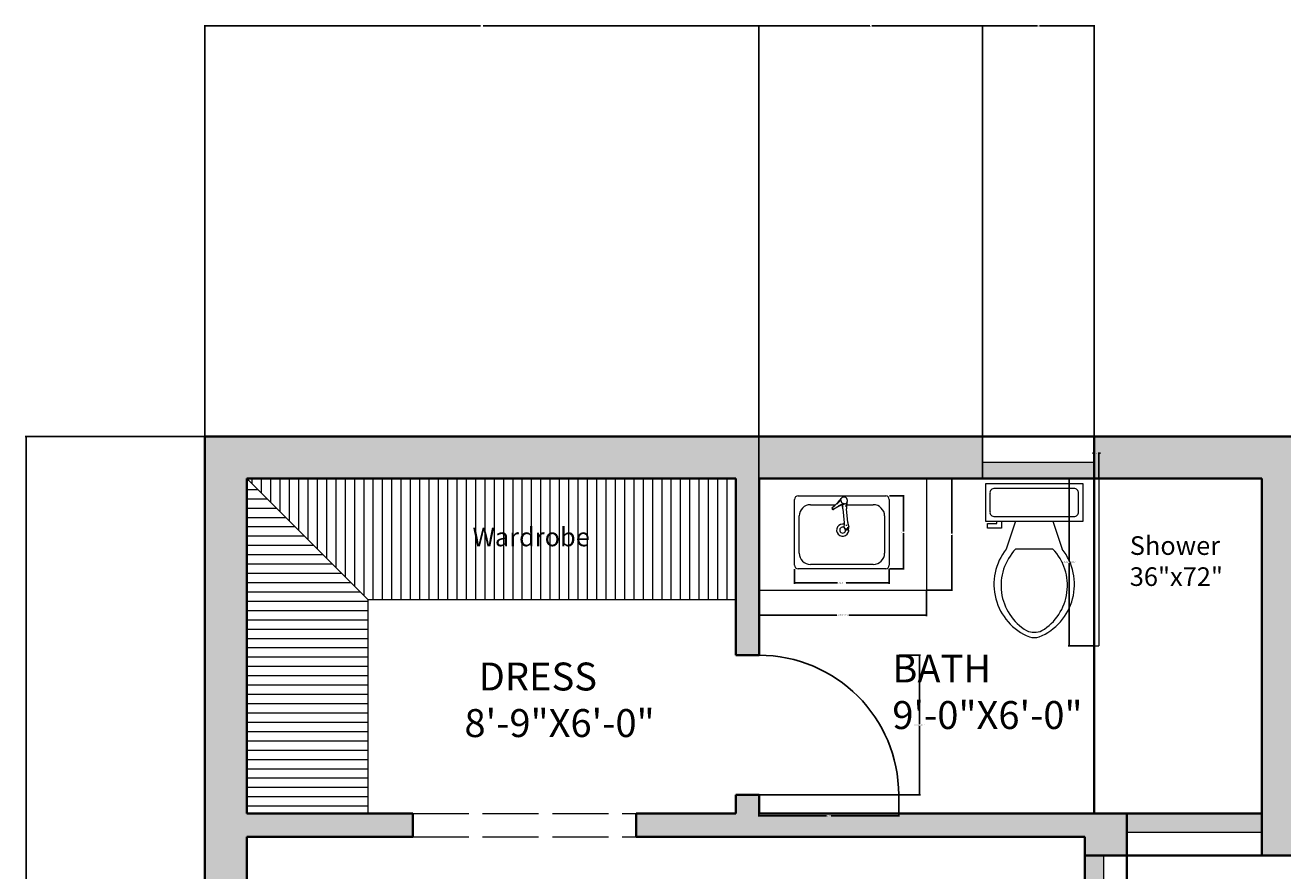
# Model space of a CAD drawing. Units: inches. Extents: x 2985 to 3527, y 3685 to 4528.
# Tile 4 of 5: x 2985 to 3255, y 4346 to 4528. Entities that reach past the tile are written whole.
import ezdxf

# ---------------------------------------------------------------- set-up
doc = ezdxf.new("R2010")
doc.units = ezdxf.units.IN
doc.linetypes.add('ACAD_ISO02W100', pattern=[15, 12, -3])
for name, color, linetype, lineweight in [('A-ANNO-DIMS', 2, 'Continuous', 18), ('A-ANNO-TEXT', 7, 'Continuous', 18), ('A-AREA-IDEN', 7, 'Continuous', 25), ('A-FLOR-CASE', 9, 'Continuous', 20), ('A-FLOR-CASE-PATT', 9, 'Continuous', 13), ('A-FLOR-FIXT', 9, 'Continuous', 18), ('A-GLAZ', 4, 'Continuous', 18), ('A-WALL', 7, 'Continuous', 40), ('A-WALL-OVHD', 7, 'ACAD_ISO02W100', 18), ('A-WALL-PATT', 8, 'Continuous', 13), ('door', 4, 'Continuous', 25)]:
    doc.layers.add(name, color=color, linetype=linetype, lineweight=lineweight)
doc.layers.add('A-GLAZ-PATT', color=241, linetype='Continuous', lineweight=13, true_color=0xf7abae)
doc.styles.get("Standard").update_dxf_attribs({"font": 'arial.ttf'})
doc.dimstyles.get("Standard").update_dxf_attribs({"dimtxt": 0.18, "dimasz": 0.18, "dimexe": 0.18, "dimexo": 0.0625, "dimgap": 0.09, "dimtad": 0, "dimtih": 1, "dimtoh": 1, "dimdec": 4, "dimzin": 0, "dimdsep": 46, "dimtxsty": 'Standard', "dimcen": 0.09, "dimadec": 0, "dimazin": 0, "dimtfac": 1, "dimtdec": 4, "dimtofl": 0, "dimtmove": 0, "dimatfit": 3, "dimfxl": 1, "dimtolj": 1, "dimtzin": 0, "dimarcsym": 0})

# ---------------------------------------------------------------- blocks, each defined once
blk = doc.blocks.new('*U2')
for p, q in [((9.5, -6), (9.5, -2)), ((-8, -8.5), (-8, -8)), ((-7, -8), (-7, -9.5)), ((-4, -8), (-6, -14)), ((4, -8), (6, -14)), ((-10, -8.5), (-8, -8.5)), ((-10, -9.5), (-10, -8.5)), ((-7, -9.5), (-10, -9.5)), ((4, -14), (-4, -14))]:
    blk.add_line(p, q)
blk.add_lwpolyline([(10.5, -8), (10.5, 0), (-10.5, 0), (-10.5, -8)], close=True)
for points in [[(-9.5, -2), (-9.5, -6)], [(8.5, -1), (-8.5, -1)], [(-8.5, -7), (8.5, -7)]]:
    blk.add_lwpolyline(points)
for centre, radius, start, end in [((-8.62, -1.88), 0.884, 81.8699, 188.1301), ((8.62, -1.88), 0.884, 351.8699, 98.1301), ((-8.62, -6.12), 0.884, 171.8699, 278.1301), ((8.62, -6.12), 0.884, 261.8699, 8.1301), ((3.52, -21.58), 12.17, 141.4691, 247.9714), ((4.2, -21.82), 11.33, 136.3677, 238.9468), ((-3.52, -21.58), 12.17, 292.0284, 38.5307), ((-4.2, -21.82), 11.33, 301.053, 43.6321), ((0, -27.88), 4, 245.7318, 294.2682), ((0, -29), 4, 254.8605, 285.1395)]:
    blk.add_arc(centre, radius, start, end)
blk = doc.blocks.new('A$C1B254B08')
for p, q in [((0, 20), (0, 394.5)), ((20, 414.5), (278.5, 414.5)), ((90.2, 364.5), (232.9, 364.5)), ((278.5, 414.5), (518, 414.5)), ((296.4, 364.5), (447.8, 364.5)), ((538, 394.5), (538, 20)), ((26.2, 88.5), (26.2, 300.5)), ((275, 340.3), (282.6, 261.9)), ((303, 263.9), (295.5, 341.4)), ((511.8, 300.5), (511.8, 88.5)), ((447.8, 24.5), (90.2, 24.5)), ((518, 0), (20, 0))]:
    blk.add_line(p, q)
for centre, radius, start, end in [((20, 394.5), 20, 90, 180), ((90.2, 300.5), 64, 90, 180), ((59.9, 551.8), 255, 307.29995, 323.44123), ((362.9, 125.6), 255, 107.37848, 123.51976), ((189.9, 438.1), 86.6, 305.66886, 327.17012), ((298.2, 285.8), 86.6, 103.6496, 125.15085), ((280, 388.4), 16.2, 164.00843, 277.23501), ((280.7, 388), 20, 287.37848, 143.44123), ((175.5, 330.4), 100, 5.6774, 19.04527), ((246.9, 349.5), 29.3, 4.17107, 27.91331), ((320.7, 356.3), 29.3, 157.81042, 186.31744), ((395, 351.3), 100, 162.19035, 185.67746), ((447.8, 300.5), 64, 0, 90), ((518, 394.5), 20, 0, 90), ((218.4, 343.7), 6.64, 127.29995, 303.51976), ((220.3, 343.9), 4.91, 158.92924, 241.9125), ((273.7, 220.2), 34.6, 74.3543, 12.13808), ((273.7, 220.2), 16.8, 61.4601, 4.85789), ((295.6, 234.6), 13.9, 171.17496, 20.1799), ((183.1, 252), 100, 351.17496, 5.6774), ((295.7, 235), 8.12, 213.71984, 15.80061), ((295.2, 239.5), 7.59, 64.48838, 123.74119), ((402.5, 273.8), 100, 185.67746, 200.1799), ((90.2, 88.5), 64, 180, 270), ((447.8, 88.5), 64, 270, 0), ((20, 20), 20, 180, 270), ((518, 20), 20, 270, 0)]:
    blk.add_arc(centre, radius, start, end)
blk = doc.blocks.new('DOOR-SWING-30IN')
blk.add_line((0, 0), (30, 0))
blk.add_arc((0, 0), 30, 0, 90)
blk = doc.blocks.new('SHOWER-SCREEN-36IN')
for p in [(1, 36), (0, 0)]:
    blk.add_line(p, (1, 0))
blk = doc.blocks.new('VANITY-TOP-36X24IN')
for p in [(36, 24), (0, 0)]:
    blk.add_line(p, (36, 0))
blk = doc.blocks.new('*D20')
at = {"layer": 'A-ANNO-DIMS', "color": 0, "lineweight": -2, "transparency": 16777216}
for p, q in [((3172.9, 4392.37), (3177.51, 4392.37)), ((3177.33, 4392.19), (3177.33, 4377.56)), ((3177.33, 4362.55), (3177.33, 4377.19)), ((3172.9, 4362.37), (3177.51, 4362.37))]:
    blk.add_line(p, q, dxfattribs=at)
at = {"layer": 'A-ANNO-DIMS', "color": 0, "transparency": 16777216}
for points in [[(3177.3, 4392.19), (3177.36, 4392.19), (3177.33, 4392.37)], [(3177.3, 4362.55), (3177.36, 4362.55), (3177.33, 4362.37)]]:
    blk.add_solid(points, dxfattribs=at)
at = {"layer": 'Defpoints', "color": 0, "transparency": 16777216}
for p in [(3172.83, 4392.37), (3177.33, 4392.37), (3172.83, 4362.37)]:
    blk.add_point(p, dxfattribs=at)
at = {"layer": 'A-ANNO-DIMS', "color": 0, "transparency": 16777216, "insert": (3177.33, 4377.37), "char_height": 0.18, "attachment_point": 5}
blk.add_mtext('\\A1;BATH DOOR 30 TYP.', dxfattribs=at)
blk = doc.blocks.new('*D21')
at = {"layer": 'A-ANNO-DIMS', "color": 0, "lineweight": -2, "transparency": 16777216}
for p, q in [((3142.83, 4362.31), (3142.83, 4357.69)), ((3172.83, 4362.31), (3172.83, 4357.69)), ((3143.01, 4357.87), (3157.31, 4357.87)), ((3172.65, 4357.87), (3158.36, 4357.87))]:
    blk.add_line(p, q, dxfattribs=at)
at = {"layer": 'A-ANNO-DIMS', "color": 0, "transparency": 16777216}
for points in [[(3143.01, 4357.9), (3143.01, 4357.84), (3142.83, 4357.87)], [(3172.65, 4357.9), (3172.65, 4357.84), (3172.83, 4357.87)]]:
    blk.add_solid(points, dxfattribs=at)
at = {"layer": 'Defpoints', "color": 0, "transparency": 16777216}
for p in [(3142.83, 4362.37), (3172.83, 4362.37), (3172.83, 4357.87)]:
    blk.add_point(p, dxfattribs=at)
at = {"layer": 'A-ANNO-DIMS', "color": 0, "transparency": 16777216, "insert": (3157.83, 4357.87), "char_height": 0.18, "attachment_point": 5}
blk.add_mtext('\\A1;30 TYP.', dxfattribs=at)
blk = doc.blocks.new('*D22')
at = {"layer": 'A-ANNO-DIMS', "color": 0, "lineweight": -2, "transparency": 16777216}
for p, q in [((3150.47, 4410.88), (3150.47, 4407.72)), ((3170.79, 4410.88), (3170.79, 4407.72)), ((3150.65, 4407.9), (3159.69, 4407.9)), ((3170.61, 4407.9), (3161.56, 4407.9))]:
    blk.add_line(p, q, dxfattribs=at)
at = {"layer": 'A-ANNO-DIMS', "color": 0, "transparency": 16777216}
for points in [[(3150.65, 4407.93), (3150.65, 4407.87), (3150.47, 4407.9)], [(3170.61, 4407.93), (3170.61, 4407.87), (3170.79, 4407.9)]]:
    blk.add_solid(points, dxfattribs=at)
at = {"layer": 'Defpoints', "color": 0, "transparency": 16777216}
for p in [(3150.47, 4410.95), (3170.79, 4410.95), (3170.79, 4407.9)]:
    blk.add_point(p, dxfattribs=at)
at = {"layer": 'A-ANNO-DIMS', "color": 0, "transparency": 16777216, "insert": (3160.63, 4407.9), "char_height": 0.18, "attachment_point": 5}
blk.add_mtext('\\A1;BASIN 20 TYP.', dxfattribs=at)
blk = doc.blocks.new('*D23')
at = {"layer": 'A-ANNO-DIMS', "color": 0, "lineweight": -2, "transparency": 16777216}
for p, q in [((3170.85, 4426.61), (3174.02, 4426.61)), ((3173.84, 4426.43), (3173.84, 4418.96)), ((3173.84, 4411.13), (3173.84, 4418.59)), ((3170.85, 4410.95), (3174.02, 4410.95))]:
    blk.add_line(p, q, dxfattribs=at)
at = {"layer": 'A-ANNO-DIMS', "color": 0, "transparency": 16777216}
for points in [[(3173.81, 4426.43), (3173.87, 4426.43), (3173.84, 4426.61)], [(3173.81, 4411.13), (3173.87, 4411.13), (3173.84, 4410.95)]]:
    blk.add_solid(points, dxfattribs=at)
at = {"layer": 'Defpoints', "color": 0, "transparency": 16777216}
for p in [(3170.79, 4426.61), (3173.84, 4426.61), (3170.79, 4410.95)]:
    blk.add_point(p, dxfattribs=at)
at = {"layer": 'A-ANNO-DIMS', "color": 0, "transparency": 16777216, "insert": (3173.84, 4418.78), "char_height": 0.18, "attachment_point": 5}
blk.add_mtext('\\A1;16 TYP.', dxfattribs=at)
blk = doc.blocks.new('*D26')
at = {"layer": 'A-ANNO-DIMS', "color": 0, "lineweight": -2, "transparency": 16777216}
for p, q in [((3214.77, 4430.37), (3209.25, 4430.37)), ((3209.43, 4430.19), (3209.43, 4412.56)), ((3209.43, 4394.55), (3209.43, 4412.19)), ((3214.77, 4394.37), (3209.25, 4394.37))]:
    blk.add_line(p, q, dxfattribs=at)
at = {"layer": 'A-ANNO-DIMS', "color": 0, "transparency": 16777216}
for points in [[(3209.4, 4430.19), (3209.46, 4430.19), (3209.43, 4430.37)], [(3209.4, 4394.55), (3209.46, 4394.55), (3209.43, 4394.37)]]:
    blk.add_solid(points, dxfattribs=at)
at = {"layer": 'Defpoints', "color": 0, "transparency": 16777216}
for p in [(3209.43, 4430.37), (3214.83, 4430.37), (3214.83, 4394.37)]:
    blk.add_point(p, dxfattribs=at)
at = {"layer": 'A-ANNO-DIMS', "color": 0, "transparency": 16777216, "insert": (3209.43, 4412.37), "char_height": 0.18, "attachment_point": 5}
blk.add_mtext('\\A1;SHOWER SCREEN 36 TYP.', dxfattribs=at)
blk = doc.blocks.new('*D27')
at = {"layer": 'A-ANNO-DIMS', "color": 0, "lineweight": -2, "transparency": 16777216}
for p, q in [((3214.65, 4435.77), (3214.47, 4435.77)), ((3214.83, 4430.43), (3214.83, 4435.95)), ((3215.83, 4430.43), (3215.83, 4435.95)), ((3216.01, 4435.77), (3216.19, 4435.77))]:
    blk.add_line(p, q, dxfattribs=at)
at = {"layer": 'A-ANNO-DIMS', "color": 0, "transparency": 16777216}
for points in [[(3214.65, 4435.8), (3214.65, 4435.74), (3214.83, 4435.77)], [(3216.01, 4435.8), (3216.01, 4435.74), (3215.83, 4435.77)]]:
    blk.add_solid(points, dxfattribs=at)
at = {"layer": 'Defpoints', "color": 0, "transparency": 16777216}
for p in [(3215.83, 4435.77), (3214.83, 4430.37), (3215.83, 4430.37)]:
    blk.add_point(p, dxfattribs=at)
at = {"layer": 'A-ANNO-DIMS', "color": 0, "transparency": 16777216, "insert": (3215.33, 4435.77), "char_height": 0.18, "attachment_point": 5}
blk.add_mtext('\\A1;1 TYP.', dxfattribs=at)
blk = doc.blocks.new('*D28')
at = {"layer": 'A-ANNO-DIMS', "color": 0, "lineweight": -2, "transparency": 16777216}
for p, q in [((3142.83, 4406.31), (3142.83, 4400.79)), ((3178.83, 4406.31), (3178.83, 4400.79)), ((3143.01, 4400.97), (3159.52, 4400.97)), ((3178.65, 4400.97), (3162.15, 4400.97))]:
    blk.add_line(p, q, dxfattribs=at)
at = {"layer": 'A-ANNO-DIMS', "color": 0, "transparency": 16777216}
for points in [[(3143.01, 4401), (3143.01, 4400.94), (3142.83, 4400.97)], [(3178.65, 4401), (3178.65, 4400.94), (3178.83, 4400.97)]]:
    blk.add_solid(points, dxfattribs=at)
at = {"layer": 'Defpoints', "color": 0, "transparency": 16777216}
for p in [(3142.83, 4406.37), (3178.83, 4406.37), (3178.83, 4400.97)]:
    blk.add_point(p, dxfattribs=at)
at = {"layer": 'A-ANNO-DIMS', "color": 0, "transparency": 16777216, "insert": (3160.83, 4400.97), "char_height": 0.18, "attachment_point": 5}
blk.add_mtext('\\A1;VANITY TOP 36 TYP.', dxfattribs=at)
blk = doc.blocks.new('*D29')
at = {"layer": 'A-ANNO-DIMS', "color": 0, "lineweight": -2, "transparency": 16777216}
for p, q in [((3178.9, 4430.37), (3184.41, 4430.37)), ((3184.23, 4430.19), (3184.23, 4418.55)), ((3184.23, 4406.55), (3184.23, 4418.19)), ((3178.9, 4406.37), (3184.41, 4406.37))]:
    blk.add_line(p, q, dxfattribs=at)
at = {"layer": 'A-ANNO-DIMS', "color": 0, "transparency": 16777216}
for points in [[(3184.2, 4430.19), (3184.26, 4430.19), (3184.23, 4430.37)], [(3184.2, 4406.55), (3184.26, 4406.55), (3184.23, 4406.37)]]:
    blk.add_solid(points, dxfattribs=at)
at = {"layer": 'Defpoints', "color": 0, "transparency": 16777216}
for p in [(3178.83, 4430.37), (3184.23, 4430.37), (3178.83, 4406.37)]:
    blk.add_point(p, dxfattribs=at)
at = {"layer": 'A-ANNO-DIMS', "color": 0, "transparency": 16777216, "insert": (3184.23, 4418.37), "char_height": 0.18, "attachment_point": 5}
blk.add_mtext('\\A1;24 TYP.', dxfattribs=at)
blk = doc.blocks.new('*D41')
at = {"layer": 'A-ANNO-DIMS', "color": 0, "lineweight": -2, "transparency": 16777216}
for p, q in [((3023.77, 4439.37), (2985.25, 4439.37)), ((2985.43, 4439.19), (2985.43, 4081.55)), ((2985.43, 3723.55), (2985.43, 4081.19)), ((3023.77, 3723.37), (2985.25, 3723.37))]:
    blk.add_line(p, q, dxfattribs=at)
at = {"layer": 'A-ANNO-DIMS', "color": 0, "transparency": 16777216}
for points in [[(2985.4, 4439.19), (2985.46, 4439.19), (2985.43, 4439.37)], [(2985.4, 3723.55), (2985.46, 3723.55), (2985.43, 3723.37)]]:
    blk.add_solid(points, dxfattribs=at)
at = {"layer": 'Defpoints', "color": 0, "transparency": 16777216}
for p in [(2985.43, 4439.37), (3023.83, 4439.37), (3023.83, 3723.37)]:
    blk.add_point(p, dxfattribs=at)
at = {"layer": 'A-ANNO-DIMS', "color": 0, "transparency": 16777216, "insert": (2985.43, 4081.37), "char_height": 0.18, "attachment_point": 5}
blk.add_mtext('\\A1;716', dxfattribs=at)
blk = doc.blocks.new('*D46')
at = {"layer": 'A-ANNO-DIMS', "color": 0, "lineweight": -2, "transparency": 16777216}
for p, q in [((3023.83, 4439.43), (3023.83, 4527.76)), ((3024.01, 4527.58), (3083.05, 4527.58)), ((3142.65, 4527.58), (3083.61, 4527.58)), ((3142.83, 4430.43), (3142.83, 4527.76))]:
    blk.add_line(p, q, dxfattribs=at)
at = {"layer": 'A-ANNO-DIMS', "color": 0, "transparency": 16777216}
for points in [[(3024.01, 4527.61), (3024.01, 4527.55), (3023.83, 4527.58)], [(3142.65, 4527.61), (3142.65, 4527.55), (3142.83, 4527.58)]]:
    blk.add_solid(points, dxfattribs=at)
at = {"layer": 'Defpoints', "color": 0, "transparency": 16777216}
for p in [(3142.83, 4527.58), (3023.83, 4439.37), (3142.83, 4430.37)]:
    blk.add_point(p, dxfattribs=at)
at = {"layer": 'A-ANNO-DIMS', "color": 0, "transparency": 16777216, "insert": (3083.33, 4527.58), "char_height": 0.18, "attachment_point": 5}
blk.add_mtext('\\A1;119', dxfattribs=at)
blk = doc.blocks.new('*D47')
at = {"layer": 'A-ANNO-DIMS', "color": 0, "lineweight": -2, "transparency": 16777216}
for p, q in [((3190.83, 4439.43), (3190.83, 4527.76)), ((3191.01, 4527.58), (3202.61, 4527.58)), ((3214.65, 4527.58), (3203.05, 4527.58)), ((3214.83, 4439.43), (3214.83, 4527.76))]:
    blk.add_line(p, q, dxfattribs=at)
at = {"layer": 'A-ANNO-DIMS', "color": 0, "transparency": 16777216}
for points in [[(3191.01, 4527.61), (3191.01, 4527.55), (3190.83, 4527.58)], [(3214.65, 4527.61), (3214.65, 4527.55), (3214.83, 4527.58)]]:
    blk.add_solid(points, dxfattribs=at)
at = {"layer": 'Defpoints', "color": 0, "transparency": 16777216}
for p in [(3214.83, 4527.58), (3190.83, 4439.37), (3214.83, 4439.37)]:
    blk.add_point(p, dxfattribs=at)
at = {"layer": 'A-ANNO-DIMS', "color": 0, "transparency": 16777216, "insert": (3202.83, 4527.58), "char_height": 0.18, "attachment_point": 5}
blk.add_mtext('\\A1;24', dxfattribs=at)
blk = doc.blocks.new('*D50')
at = {"layer": 'A-ANNO-DIMS', "color": 0, "lineweight": -2, "transparency": 16777216}
for p, q in [((3142.83, 4430.43), (3142.83, 4527.76)), ((3143.01, 4527.58), (3166.61, 4527.58)), ((3190.65, 4527.58), (3167.06, 4527.58)), ((3190.83, 4430.43), (3190.83, 4527.76))]:
    blk.add_line(p, q, dxfattribs=at)
at = {"layer": 'A-ANNO-DIMS', "color": 0, "transparency": 16777216}
for points in [[(3143.01, 4527.61), (3143.01, 4527.55), (3142.83, 4527.58)], [(3190.65, 4527.61), (3190.65, 4527.55), (3190.83, 4527.58)]]:
    blk.add_solid(points, dxfattribs=at)
at = {"layer": 'Defpoints', "color": 0, "transparency": 16777216}
for p in [(3190.83, 4527.58), (3142.83, 4430.37), (3190.83, 4430.37)]:
    blk.add_point(p, dxfattribs=at)
at = {"layer": 'A-ANNO-DIMS', "color": 0, "transparency": 16777216, "insert": (3166.83, 4527.58), "char_height": 0.18, "attachment_point": 5}
blk.add_mtext('\\A1;48', dxfattribs=at)

msp = doc.modelspace()

# ---------------------------------------------------------------- hatches: boundary and pattern name
at = {"layer": 'A-FLOR-CASE-PATT'}
h = msp.add_hatch(dxfattribs=at)
h.set_pattern_fill('ANSI31', color=256, scale=0.6299213, angle=-45, style=0)
h.paths.add_polyline_path([(3032.833, 4358.372), (3058.833, 4358.372), (3058.833, 4404.372), (3032.833, 4430.372)])
h = msp.add_hatch(dxfattribs=at)
h.set_pattern_fill('ANSI31', color=256, scale=0.6299213, angle=45, style=0)
h.paths.add_polyline_path([(3032.833, 4430.372), (3058.833, 4404.372), (3137.833, 4404.372), (3137.833, 4430.372)])
at = {"layer": 'A-GLAZ-PATT'}
h = msp.add_hatch(color=256, dxfattribs=at)
h.dxf.hatch_style = 1
h.paths.add_polyline_path([(3214.833, 4433.872), (3190.833, 4433.872), (3190.833, 4430.372), (3214.833, 4430.372)])
h = msp.add_hatch(color=256, dxfattribs=at)
h.dxf.hatch_style = 1
h.paths.add_polyline_path([(3216.833, 4349.372), (3212.833, 4349.372), (3212.833, 4271.372), (3216.833, 4271.372)])
h.paths.add_polyline_path([(3250.833, 4358.372), (3221.833, 4358.372), (3221.833, 4354.372), (3250.833, 4354.372)])
h.paths.add_polyline_path([(3290.333, 4358.372), (3259.833, 4358.372), (3259.833, 4354.372), (3290.333, 4354.372)])
h.paths.add_polyline_path([(3299.333, 4349.372), (3295.333, 4349.372), (3295.333, 4271.372), (3299.333, 4271.372)])
h.paths.add_polyline_path([(3290.333, 4265.372), (3221.833, 4265.372), (3221.833, 4260.372), (3290.333, 4260.372)])
at = {"layer": 'A-WALL-PATT'}
h = msp.add_hatch(color=256, dxfattribs=at)
h.dxf.hatch_style = 1
h.paths.add_polyline_path([(3023.833, 4065.372), (3023.833, 3771.372), (3111.083, 3771.372), (3111.083, 3780.372), (3032.833, 3780.372), (3032.833, 3936.372), (3221.333, 3936.372), (3221.333, 3945.372), (3215.333, 3945.372), (3215.333, 3981.372), (3206.333, 3981.372), (3206.333, 3945.372), (3032.833, 3945.372), (3032.833, 4065.372), (3079.333, 4065.372), (3079.333, 4074.372), (3032.833, 4074.372), (3032.833, 4188.372), (3119.333, 4188.372), (3119.333, 4107.372), (3215.333, 4107.372), (3215.333, 4148.372), (3206.333, 4148.372), (3206.333, 4116.372), (3124.333, 4116.372), (3124.333, 4188.372), (3206.333, 4188.372), (3206.333, 4184.372), (3215.333, 4184.372), (3215.333, 4188.372), (3221.833, 4188.372), (3221.833, 4201.372), (3212.833, 4201.372), (3212.833, 4197.372), (3032.833, 4197.372), (3032.833, 4353.372), (3068.479, 4353.372), (3068.479, 4358.372), (3032.833, 4358.372), (3032.833, 4430.372), (3137.833, 4430.372), (3137.833, 4404.372), (3137.833, 4392.372), (3142.833, 4392.372), (3142.833, 4430.372), (3190.833, 4430.372), (3190.833, 4439.372), (3023.833, 4439.372)])
h = msp.add_hatch(color=256, dxfattribs=at)
h.dxf.hatch_style = 1
h.paths.add_polyline_path([(3259.833, 4430.372), (3295.833, 4430.372), (3295.833, 4439.372), (3214.833, 4439.372), (3214.833, 4430.372), (3250.833, 4430.372), (3250.833, 4349.372), (3259.833, 4349.372)])
h = msp.add_hatch(color=256, dxfattribs=at)
h.dxf.hatch_style = 1
h.paths.add_polyline_path([(3221.833, 4358.372), (3142.833, 4358.372), (3142.833, 4362.372), (3137.833, 4362.372), (3137.833, 4358.372), (3116.479, 4358.372), (3116.479, 4353.372), (3212.833, 4353.372), (3212.833, 4349.372), (3221.833, 4349.372)])

# ---------------------------------------------------------------- linework, layer by layer
at = {"layer": 'A-FLOR-CASE'}
for q in [(3032.833, 4430.372), (3137.833, 4404.372), (3058.833, 4358.372)]:
    msp.add_line((3058.833, 4404.372), q, dxfattribs=at)
at = {"layer": 'A-GLAZ'}
for p, q in [((3190.833, 4439.372), (3190.833, 4430.372)), ((3190.833, 4433.872), (3214.833, 4433.872)), ((3221.833, 4354.372), (3250.833, 4354.372)), ((3216.833, 4349.372), (3216.833, 4271.372))]:
    msp.add_line(p, q, dxfattribs=at)
at = {"layer": 'A-WALL'}
for p, q in [((3023.833, 4439.372), (3023.833, 4065.372)), ((3023.833, 4439.372), (3488.333, 4439.372)), ((3214.833, 4439.372), (3214.833, 4358.372)), ((3032.833, 4430.372), (3032.833, 4358.372)), ((3032.833, 4430.372), (3137.833, 4430.372)), ((3137.833, 4430.372), (3137.833, 4404.372)), ((3142.833, 4430.372), (3142.833, 4392.372)), ((3142.833, 4430.372), (3250.833, 4430.372)), ((3250.833, 4430.372), (3250.833, 4349.372)), ((3137.833, 4404.372), (3137.833, 4392.372)), ((3142.833, 4392.372), (3137.833, 4392.372)), ((3142.833, 4362.372), (3137.833, 4362.372)), ((3137.833, 4362.372), (3137.833, 4358.372)), ((3142.833, 4362.372), (3142.833, 4358.372)), ((3032.833, 4358.372), (3068.479, 4358.372)), ((3068.479, 4358.372), (3068.479, 4353.372)), ((3116.479, 4358.372), (3116.479, 4353.372)), ((3116.479, 4358.372), (3137.833, 4358.372)), ((3142.833, 4358.372), (3250.833, 4358.372)), ((3221.833, 4358.372), (3221.833, 4237.372)), ((3032.833, 4353.372), (3068.479, 4353.372)), ((3032.833, 4353.372), (3032.833, 4197.372)), ((3116.479, 4353.372), (3212.833, 4353.372)), ((3212.833, 4353.372), (3212.833, 4237.372)), ((3212.833, 4349.372), (3299.333, 4349.372))]:
    msp.add_line(p, q, dxfattribs=at)
at = {"layer": 'A-WALL-OVHD'}
for p, q in [((3068.479, 4358.372), (3116.479, 4358.372)), ((3068.479, 4353.372), (3116.479, 4353.372))]:
    msp.add_line(p, q, dxfattribs=at)

# ---------------------------------------------------------------- block references
at = {"layer": 'A-FLOR-CASE'}
msp.add_blockref('VANITY-TOP-36X24IN', (3142.833, 4406.372), dxfattribs=at)
at = {"layer": 'A-FLOR-FIXT'}
for name, p in [('SHOWER-SCREEN-36IN', (3214.833, 4394.372)), ('*U2', (3201.94, 4429.183))]:
    msp.add_blockref(name, p, dxfattribs=at)
at = {"layer": 'A-FLOR-FIXT', "xscale": 0.0377799968595654, "yscale": 0.0377799968595654, "zscale": 0.0377799968595654}
msp.add_blockref('A$C1B254B08', (3150.465, 4410.947), dxfattribs=at)
at = {"layer": 'door'}
msp.add_blockref('DOOR-SWING-30IN', (3142.833, 4362.372), dxfattribs=at)

# ---------------------------------------------------------------- texts
at = {"layer": 'A-ANNO-TEXT', "char_height": 4, "attachment_point": 1}
for s, width, insert in [('Wardrobe', 30.56793, (3081.313, 4419.784)), ('Shower\\P36"x72"', 18.2759, (3222.46, 4417.934))]:
    msp.add_mtext_dynamic_manual_height_columns(s, width=width, gutter_width=12.5, heights=[0], dxfattribs=dict(at, insert=insert))
at = {"layer": 'A-AREA-IDEN', "attachment_point": 1}
for s, width, insert, char_height in [('BATH\\P9\'-0"X6\'-0"', 24.98129, (3171.463, 4392.524), 6), ('    {\\H2.4x;DRESS\\P8\'-9"X6\'-0"}', 78.32659, (3079.571, 4390.8), 2.5)]:
    msp.add_mtext_dynamic_manual_height_columns(s, width=width, gutter_width=12.5, heights=[0], dxfattribs=dict(at, insert=insert, char_height=char_height))

# ---------------------------------------------------------------- dimensions: what is measured, and where the dimension line sits
at = {"layer": 'A-ANNO-DIMS'}
for base, p1, p2, picture, middle in [((3142.833, 4527.583), (3023.833, 4439.372), (3142.833, 4430.372), '*D46', (3083.333, 4527.583)), ((3190.833, 4527.583), (3142.833, 4430.372), (3190.833, 4430.372), '*D50', (3166.833, 4527.583)), ((3214.833, 4527.583), (3190.833, 4439.372), (3214.833, 4439.372), '*D47', (3202.833, 4527.583))]:
    dim = msp.add_linear_dim(base=base, p1=p1, p2=p2, dimstyle='Standard', override={"dimdec": 0, "dimlfac": 1, "dimrnd": 0, "dimzin": 0, "dimdsep": 46, "dimlunit": 2}, dxfattribs=at)
    dim.commit()
    dim.dimension.update_dxf_attribs({"geometry": picture, "text_midpoint": middle})
dim = msp.add_linear_dim(base=(2985.433, 4439.372), p1=(3023.833, 3723.372), p2=(3023.833, 4439.372), angle=90, dimstyle='Standard', override={"dimdec": 0, "dimlfac": 1, "dimrnd": 0, "dimzin": 0, "dimdsep": 46, "dimlunit": 2}, dxfattribs=at)
dim.commit()
dim.dimension.update_dxf_attribs({"geometry": '*D41', "text_midpoint": (2985.433, 4081.372)})
for base, p1, p2, text, picture, middle in [((3215.833, 4435.772), (3214.833, 4430.372), (3215.833, 4430.372), '<> TYP.', '*D27', (3215.333, 4435.772)), ((3170.792, 4407.898), (3150.465, 4410.947), (3170.792, 4410.947), 'BASIN <> TYP.', '*D22', (3160.628, 4407.898)), ((3178.833, 4400.972), (3142.833, 4406.372), (3178.833, 4406.372), 'VANITY TOP <> TYP.', '*D28', (3160.833, 4400.972)), ((3172.833, 4357.872), (3142.833, 4362.372), (3172.833, 4362.372), '<> TYP.', '*D21', (3157.833, 4357.872))]:
    dim = msp.add_linear_dim(base=base, p1=p1, p2=p2, text=text, dimstyle='Standard', override={"dimdec": 0, "dimlfac": 1, "dimrnd": 0, "dimzin": 0, "dimdsep": 46, "dimlunit": 2}, dxfattribs=at)
    dim.commit()
    dim.dimension.update_dxf_attribs({"geometry": picture, "text_midpoint": middle})
for base, p1, p2, text, picture, middle in [((3184.233, 4430.372), (3178.833, 4406.372), (3178.833, 4430.372), '<> TYP.', '*D29', (3184.233, 4418.372)), ((3209.433, 4430.372), (3214.833, 4394.372), (3214.833, 4430.372), 'SHOWER SCREEN <> TYP.', '*D26', (3209.433, 4412.372)), ((3173.841, 4426.606), (3170.792, 4410.947), (3170.792, 4426.606), '<> TYP.', '*D23', (3173.841, 4418.776)), ((3177.333, 4392.372), (3172.833, 4362.372), (3172.833, 4392.372), 'BATH DOOR <> TYP.', '*D20', (3177.333, 4377.372))]:
    dim = msp.add_linear_dim(base=base, p1=p1, p2=p2, angle=90, text=text, dimstyle='Standard', override={"dimdec": 0, "dimlfac": 1, "dimrnd": 0, "dimzin": 0, "dimdsep": 46, "dimlunit": 2}, dxfattribs=at)
    dim.commit()
    dim.dimension.update_dxf_attribs({"geometry": picture, "text_midpoint": middle})

doc.saveas('drawing.dxf')
